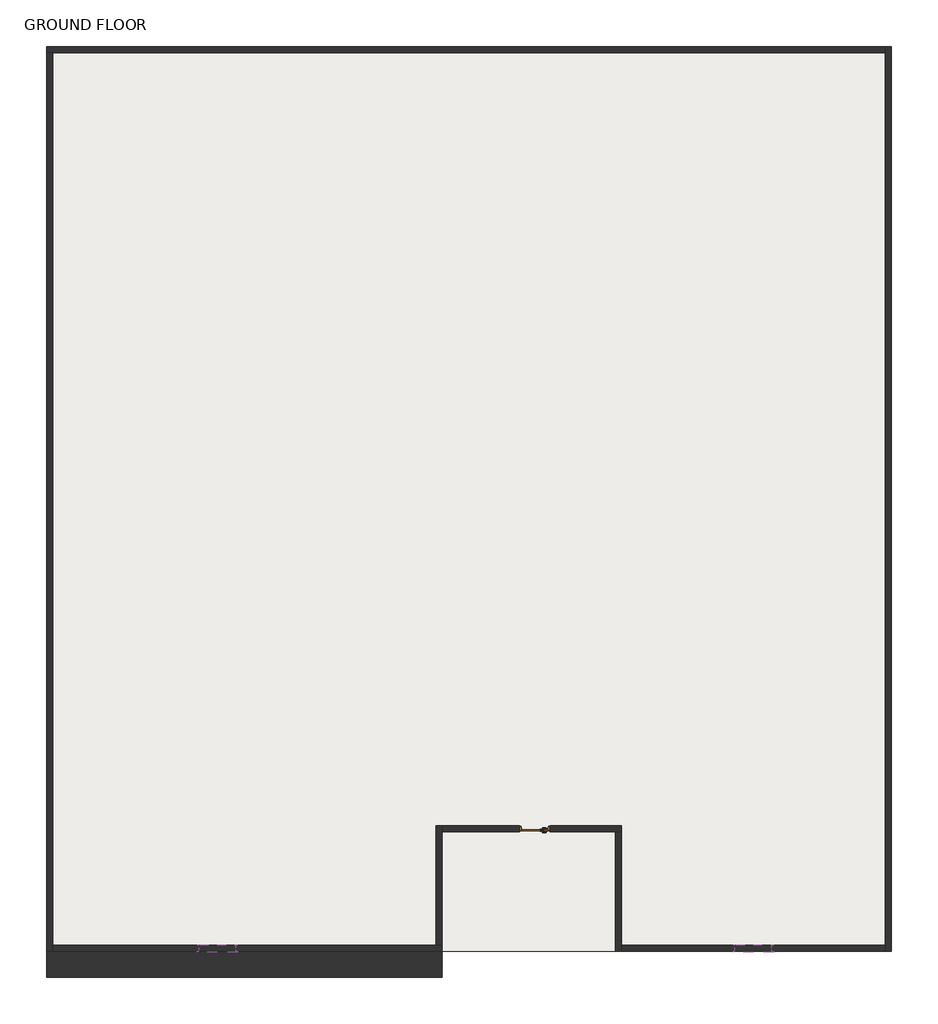
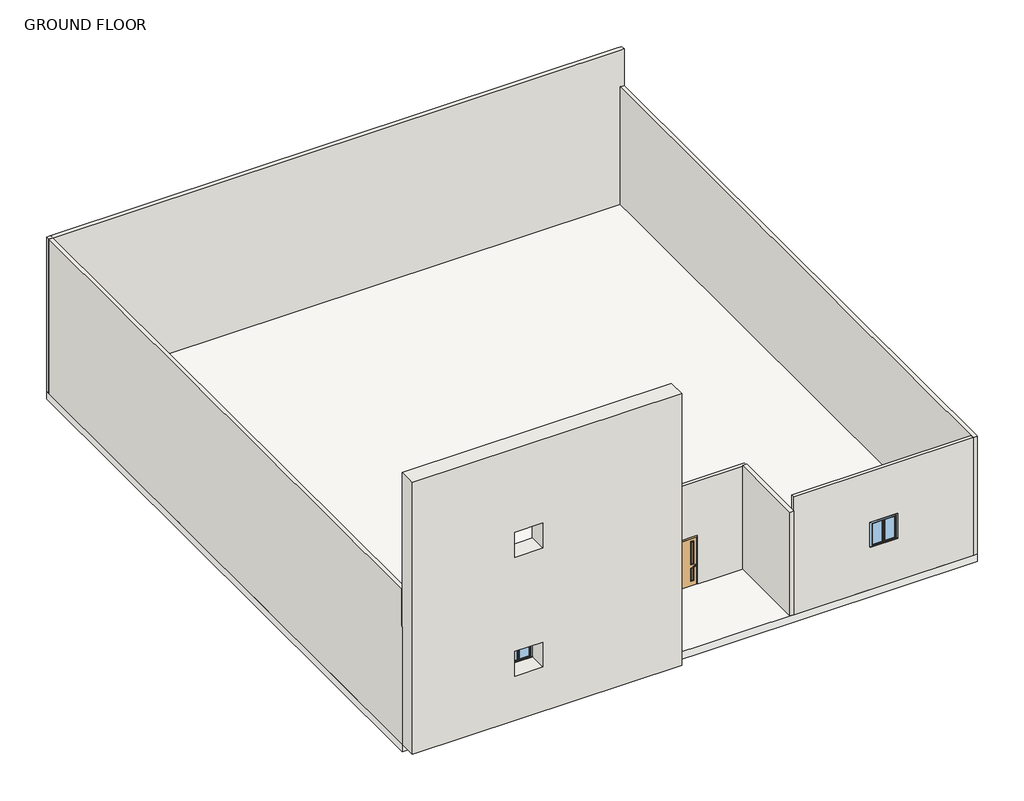
# One storey: 12 walls, 2 slabs, 2 windows, 1 door.
"""IFC4 building model written with IfcOpenShell, lengths in millimetres."""

from ifc_helpers import new_model, si_unit, frame, origin, place, context, project, spatial, polyline, outline, extrude, faceted_brep, transform, mapped, element, save
from components import door_81f4c142, walls_1_walls_1_ac0e2196, window_264d1730

model = new_model("IFC4")

# Units and contexts
model_context = context("Model", 3, world=origin())
ifc_project = project(units=[si_unit("LENGTHUNIT", "METRE", prefix="MILLI")], contexts=[model_context])

# Site, building, storey
site = spatial("IfcSite", under=ifc_project)
building = spatial("IfcBuilding", under=site)
storey = spatial("IfcBuildingStorey", under=building, Name="GROUND FLOOR", Elevation=0.0)

# Door
placement = place(None, origin())
door_shape = door_81f4c142(model_context)
element("IfcDoor", 1, ObjectType="Door-Passage-Single-Vision_Two_Lite : 36\" x 96\"", at=placement, inside=storey, context=model_context, shape_type="MappedRepresentation", body=[
    mapped(door_shape, transform((-1590.01982, -3826.5465627, 0.0), x_axis=(-1.0, 0.0, 0.0), y_axis=(0.0, -1.0, 0.0), z_axis=(0.0, 0.0, 1.0))),
])

# Slabs
element("IfcSlab", 2, ObjectType="Generic Floor - 400mm", at=placement, inside=storey, context=model_context, shape_type="SweptSolid", body=[
    extrude(outline(polyline([(10309.98018, 22267.1034373), (10309.98018, -7932.8965627), (-17890.01982, -7932.8965627), (-17890.01982, 22267.1034373), (10309.98018, 22267.1034373)])), frame((0.0, 0.0, -400.0), z_axis=(0.0, 0.0, 1.0), x_axis=(1.0, 0.0, 0.0)), (0.0, 0.0, 1.0), 400.0),
])
element("IfcSlab", 3, ObjectType="Generic Floor - 400mm", at=placement, inside=storey, context=model_context, shape_type="SweptSolid", body=[
    extrude(outline(polyline([(10309.98018, 22267.1034373), (10309.98018, -7932.8965627), (-17890.01982, -7932.8965627), (-17890.01982, 22267.1034373), (10309.98018, 22267.1034373)])), frame((0.0, 0.0, -400.0), z_axis=(0.0, 0.0, 1.0), x_axis=(1.0, 0.0, 0.0)), (0.0, 0.0, 1.0), 400.0),
])

# Walls
element("IfcWall", 4, ObjectType="Generic - 9\"", at=placement, inside=storey, context=model_context, shape_type="Brep", body=[
    faceted_brep([(-17890.01982, 22067.1034373, 8000.0), (-17890.01982, 22067.1034373, 6096.0), (-17890.01982, 22067.1034373, 0.0), (-17690.01982, 22067.1034373, 0.0), (10109.98018, 22067.1034373, 0.0), (10109.98018, 22067.1034373, 6096.0), (10309.98018, 22067.1034373, 6096.0), (10309.98018, 22067.1034373, 8000.0), (10109.98018, 22067.1034373, 8000.0), (-17690.01982, 22067.1034373, 8000.0), (-17890.01982, 22267.1034373, 0.0), (-17890.01982, 22267.1034373, 8000.0), (-17690.01982, 22267.1034373, 8000.0), (10109.98018, 22267.1034373, 8000.0), (10309.98018, 22267.1034373, 8000.0), (10309.98018, 22267.1034373, 6096.0), (10109.98018, 22267.1034373, 6096.0), (10109.98018, 22267.1034373, 0.0)], [[[0, 1, 2, 3, 4, 5, 6, 7, 8, 9]], [[10, 11, 12, 13, 14, 15, 16, 17]], [[4, 3, 2, 10, 17]], [[0, 9, 8, 7, 14, 13, 12, 11]], [[0, 11, 10, 2, 1]], [[15, 6, 5, 16]], [[5, 4, 17, 16]], [[7, 6, 15, 14]]]),
])
element("IfcWall", 5, ObjectType="Generic - 9\"", at=placement, inside=storey, context=model_context, shape_type="Brep", body=[
    faceted_brep([(-17690.01982, -7932.8965627, 0.0), (-17690.01982, -7732.8965627, 0.0), (-17690.01982, 22067.1034373, 0.0), (-17690.01982, 22067.1034373, 8000.0), (-17690.01982, -7832.8965627, 8000.0), (-17690.01982, -7832.8965627, 6096.0), (-17690.01982, -7932.8965627, 6096.0), (-17890.01982, -7932.8965627, 0.0), (-17890.01982, -7932.8965627, 6096.0), (-17890.01982, -7832.8965627, 6096.0), (-17890.01982, -7832.8965627, 8000.0), (-17890.01982, 22067.1034373, 8000.0), (-17890.01982, 22067.1034373, 0.0)], [[[0, 1, 2, 3, 4, 5, 6]], [[7, 8, 9, 10, 11, 12]], [[2, 1, 0, 7, 12]], [[4, 3, 11, 10]], [[5, 4, 10, 9]], [[5, 9, 8, 6]], [[0, 6, 8, 7]], [[2, 12, 11, 3]]]),
])
element("IfcWall", 6, ObjectType="Generic - 9\"", at=placement, inside=storey, context=model_context, shape_type="Brep", body=[
    faceted_brep([(10109.98018, 22267.1034373, 0.0), (10109.98018, 22067.1034373, 0.0), (10109.98018, -7732.8965627, 0.0), (10109.98018, -7932.8965627, 0.0), (10109.98018, -7932.8965627, 6096.0), (10109.98018, -7832.8965627, 6096.0), (10109.98018, -7732.8965627, 6096.0), (10109.98018, -3632.8965627, 6096.0), (10109.98018, 22067.1034373, 6096.0), (10109.98018, 22267.1034373, 6096.0), (10309.98018, 22267.1034373, 0.0), (10309.98018, 22267.1034373, 6096.0), (10309.98018, 22067.1034373, 6096.0), (10309.98018, -3632.8965627, 6096.0), (10309.98018, -7832.8965627, 6096.0), (10309.98018, -7932.8965627, 6096.0), (10309.98018, -7932.8965627, 0.0)], [[[0, 1, 2, 3, 4, 5, 6, 7, 8, 9]], [[10, 11, 12, 13, 14, 15, 16]], [[3, 2, 1, 0, 10, 16]], [[9, 8, 7, 6, 5, 4, 15, 14, 13, 12, 11]], [[0, 9, 11, 10]], [[4, 3, 16, 15]]]),
])
element("IfcWall", 7, ObjectType="Generic - 9\"", at=placement, inside=storey, context=model_context, shape_type="Brep", body=[
    faceted_brep([(-17690.01982, 22067.1034373, 8000.0), (-17690.01982, 22067.1034373, 0.0), (10109.98018, 22067.1034373, 0.0), (10109.98018, 22067.1034373, 6096.0), (10309.98018, 22067.1034373, 6096.0), (10309.98018, 22067.1034373, 8000.0), (10109.98018, 22067.1034373, 8000.0), (-17690.01982, 22267.1034373, 0.0), (-17690.01982, 22267.1034373, 8000.0), (10109.98018, 22267.1034373, 8000.0), (10309.98018, 22267.1034373, 8000.0), (10309.98018, 22267.1034373, 6096.0), (10109.98018, 22267.1034373, 6096.0), (10109.98018, 22267.1034373, 0.0)], [[[0, 1, 2, 3, 4, 5, 6]], [[7, 8, 9, 10, 11, 12, 13]], [[2, 1, 7, 13]], [[0, 6, 5, 10, 9, 8]], [[0, 8, 7, 1]], [[11, 4, 3, 12]], [[3, 2, 13, 12]], [[5, 4, 11, 10]]]),
])
element("IfcWall", 8, ObjectType="Generic - 9\"", at=placement, inside=storey, context=model_context, shape_type="Brep", body=[
    faceted_brep([(-17690.01982, -7932.8965627, 0.0), (-17690.01982, -7732.8965627, 0.0), (-17690.01982, 22067.1034373, 0.0), (-17690.01982, 22067.1034373, 8000.0), (-17690.01982, -7832.8965627, 8000.0), (-17690.01982, -7832.8965627, 6096.0), (-17690.01982, -7932.8965627, 6096.0), (-17890.01982, -7932.8965627, 0.0), (-17890.01982, -7932.8965627, 6096.0), (-17890.01982, -7832.8965627, 6096.0), (-17890.01982, -7832.8965627, 8000.0), (-17890.01982, 22067.1034373, 8000.0), (-17890.01982, 22067.1034373, 0.0)], [[[0, 1, 2, 3, 4, 5, 6]], [[7, 8, 9, 10, 11, 12]], [[2, 1, 0, 7, 12]], [[4, 3, 11, 10]], [[2, 12, 11, 3]], [[5, 4, 10, 9]], [[5, 9, 8, 6]], [[0, 6, 8, 7]]]),
])
element("IfcWall", 9, ObjectType="Generic - 9\"", at=placement, inside=storey, context=model_context, shape_type="Brep", body=[
    faceted_brep([(10109.98018, 22067.1034373, 0.0), (10109.98018, -7732.8965627, 0.0), (10109.98018, -7932.8965627, 0.0), (10109.98018, -7932.8965627, 6096.0), (10109.98018, -7832.8965627, 6096.0), (10109.98018, -7732.8965627, 6096.0), (10109.98018, -3632.8965627, 6096.0), (10109.98018, 22067.1034373, 6096.0), (10309.98018, 22067.1034373, 0.0), (10309.98018, 22067.1034373, 6096.0), (10309.98018, -3632.8965627, 6096.0), (10309.98018, -7832.8965627, 6096.0), (10309.98018, -7932.8965627, 6096.0), (10309.98018, -7932.8965627, 0.0)], [[[0, 1, 2, 3, 4, 5, 6, 7]], [[8, 9, 10, 11, 12, 13]], [[2, 1, 0, 8, 13]], [[7, 6, 5, 4, 3, 12, 11, 10, 9]], [[0, 7, 9, 8]], [[3, 2, 13, 12]]]),
])
element("IfcWall", 10, ObjectType="Generic - 9\"", at=placement, inside=storey, context=model_context, shape_type="Brep", body=[
    faceted_brep([(-17690.01982, -7932.8965627, 0.0), (-4690.01982, -7932.8965627, 0.0), (-4690.01982, -7932.8965627, 6096.0), (-4790.01982, -7932.8965627, 6096.0), (-17690.01982, -7932.8965627, 6096.0), (-12799.61982, -7932.8965627, 3545.6933591), (-11580.41982, -7932.8965627, 3545.6933591), (-11580.41982, -7932.8965627, 2326.4933591), (-12799.61982, -7932.8965627, 2326.4933591), (-17690.01982, -7732.8965627, 0.0), (-17690.01982, -7732.8965627, 6096.0), (-4790.01982, -7732.8965627, 6096.0), (-4690.01982, -7732.8965627, 6096.0), (-4690.01982, -7732.8965627, 5646.6011472), (-4690.01982, -7732.8965627, 0.0), (-4890.01982, -7732.8965627, 0.0), (-12799.61982, -7732.8965627, 3545.6933591), (-12799.61982, -7732.8965627, 2326.4933591), (-11580.41982, -7732.8965627, 2326.4933591), (-11580.41982, -7732.8965627, 3545.6933591), (-17690.01982, -7832.8965627, 6096.0)], [[[0, 1, 2, 3, 4], [5, 6, 7, 8]], [[9, 10, 11, 12, 13, 14, 15], [16, 17, 18, 19]], [[1, 0, 9, 15, 14]], [[4, 3, 2, 12, 11, 10, 20]], [[2, 1, 14, 13, 12]], [[0, 4, 20, 10, 9]], [[17, 16, 5, 8]], [[18, 17, 8, 7]], [[19, 18, 7, 6]], [[16, 19, 6, 5]]]),
])
element("IfcWall", 11, ObjectType="Generic - 9\"", at=placement, inside=storey, context=model_context, shape_type="Brep", body=[
    faceted_brep([(-4690.01982, -7732.8965627, 0.0), (-4690.01982, -3932.8965627, 0.0), (-4690.01982, -3732.8965627, 0.0), (-4690.01982, -3732.8965627, 5329.0930387), (-4690.01982, -3732.8965627, 5646.6011472), (-4690.01982, -7732.8965627, 5646.6011472), (-4890.01982, -7732.8965627, 0.0), (-4890.01982, -7732.8965627, 5646.6011472), (-4890.01982, -3732.8965627, 5646.6011472), (-4890.01982, -3732.8965627, 0.0)], [[[0, 1, 2, 3, 4, 5]], [[6, 7, 8, 9]], [[2, 1, 0, 6, 9]], [[5, 4, 8, 7]], [[0, 5, 7, 6]], [[4, 3, 2, 9, 8]]]),
])
element("IfcWall", 12, ObjectType="Generic - 9\"", at=placement, inside=storey, context=model_context, shape_type="Brep", body=[
    faceted_brep([(1309.98018, -3932.8965627, 5329.0930387), (-4690.01982, -3932.8965627, 5329.0930387), (-4690.01982, -3932.8965627, 0.0), (-2098.01982, -3932.8965627, 0.0), (-2098.01982, -3932.8965627, 2540.0), (-1082.01982, -3932.8965627, 2540.0), (-1082.01982, -3932.8965627, 0.0), (1109.98018, -3932.8965627, 0.0), (1309.98018, -3932.8965627, 0.0), (-4690.01982, -3732.8965627, 5329.0930387), (1309.98018, -3732.8965627, 5329.0930387), (1309.98018, -3732.8965627, 0.0), (-1082.01982, -3732.8965627, 0.0), (-1082.01982, -3732.8965627, 2540.0), (-2098.01982, -3732.8965627, 2540.0), (-2098.01982, -3732.8965627, 0.0), (-4690.01982, -3732.8965627, 0.0)], [[[0, 1, 2, 3, 4, 5, 6, 7, 8]], [[9, 10, 11, 12, 13, 14, 15, 16]], [[2, 16, 15, 3]], [[11, 8, 7, 6, 12]], [[1, 0, 10, 9]], [[2, 1, 9, 16]], [[0, 8, 11, 10]], [[14, 4, 3, 15]], [[4, 14, 13, 5]], [[5, 13, 12, 6]]]),
])
element("IfcWall", 13, ObjectType="Generic - 9\"", at=placement, inside=storey, context=model_context, shape_type="Brep", body=[
    faceted_brep([(1109.98018, -3932.8965627, 0.0), (1109.98018, -7932.8965627, 0.0), (1109.98018, -7932.8965627, 5381.5090557), (1109.98018, -3932.8965627, 5381.5090557), (1309.98018, -3932.8965627, 0.0), (1309.98018, -3932.8965627, 5329.0930387), (1309.98018, -3932.8965627, 5381.5090557), (1309.98018, -7932.8965627, 5381.5090557), (1309.98018, -7932.8965627, 0.0), (1309.98018, -7732.8965627, 0.0)], [[[0, 1, 2, 3]], [[4, 5, 6, 7, 8, 9]], [[1, 0, 4, 9, 8]], [[3, 2, 7, 6]], [[0, 3, 6, 5, 4]], [[2, 1, 8, 7]]]),
])
element("IfcWall", 14, ObjectType="Generic - 9\"", at=placement, inside=storey, context=model_context, shape_type="Brep", body=[
    faceted_brep([(1309.98018, -7932.8965627, 0.0), (10109.98018, -7932.8965627, 0.0), (10109.98018, -7932.8965627, 6096.0), (1309.98018, -7932.8965627, 6096.0), (1309.98018, -7932.8965627, 5381.5090557), (5100.38018, -7932.8965627, 3419.8751227), (6319.58018, -7932.8965627, 3419.8751227), (6319.58018, -7932.8965627, 2200.6751227), (5100.38018, -7932.8965627, 2200.6751227), (1309.98018, -7732.8965627, 0.0), (1309.98018, -7732.8965627, 6096.0), (10109.98018, -7732.8965627, 6096.0), (10109.98018, -7732.8965627, 0.0), (5100.38018, -7732.8965627, 3419.8751227), (5100.38018, -7732.8965627, 2200.6751227), (6319.58018, -7732.8965627, 2200.6751227), (6319.58018, -7732.8965627, 3419.8751227)], [[[0, 1, 2, 3, 4], [5, 6, 7, 8]], [[9, 10, 11, 12], [13, 14, 15, 16]], [[1, 0, 9, 12]], [[3, 2, 11, 10]], [[2, 1, 12, 11]], [[14, 13, 5, 8]], [[15, 14, 8, 7]], [[16, 15, 7, 6]], [[13, 16, 6, 5]], [[0, 4, 3, 10, 9]]]),
])
walls_1_walls_1_shape = walls_1_walls_1_ac0e2196(model_context)
element("IfcWall", 15, ObjectType="Walls 1 : Walls 1", at=placement, inside=storey, context=model_context, shape_type="MappedRepresentation", body=[
    mapped(walls_1_walls_1_shape, transform((0.0, 0.0, 0.0), x_axis=(1.0, 0.0, 0.0), y_axis=(0.0, 1.0, 0.0), z_axis=(0.0, 0.0, 1.0))),
])

# Windows
window_shape = window_264d1730(model_context)
element("IfcWindow", 16, ObjectType="Casement Dbl with Trim : 48\" x 48\"", at=placement, inside=storey, context=model_context, shape_type="MappedRepresentation", body=[
    mapped(window_shape, transform((-12190.01982, -7813.8465627, 1412.0933591), x_axis=(-1.0, 0.0, 0.0), y_axis=(0.0, -1.0, 0.0), z_axis=(0.0, 0.0, 1.0))),
])
element("IfcWindow", 17, ObjectType="Casement Dbl with Trim : 48\" x 48\"", at=placement, inside=storey, context=model_context, shape_type="MappedRepresentation", body=[
    mapped(window_shape, transform((5709.98018, -7813.8465627, 1286.2751227), x_axis=(-1.0, 0.0, 0.0), y_axis=(0.0, -1.0, 0.0), z_axis=(0.0, 0.0, 1.0))),
])

save(model, "model.ifc")

# Revit data of these elements
# Type "Door-Passage-Single-Vision_Two_Lite : 36\" x 96\""
#   Type Mark = "22"
#   Assembly Code = "B2030100"
#   Analytic Construction = "Wooden"
#   Thickness = 0' - 1 3/4"
#   Thermal Resistance (R) = 0.455703 (m²·K)/W
#   Swing Angle [instance default] = 90.00°
#   Strike Height = 3' - 4"
#   Rough Width [instance default] = 3' - 4"
#   Rough Height [instance default] = 8' - 4"
#   MF Opening Height [instance default] = 0' - 4"
#   MF Opening Width [instance default] = 0' - 4"
#   Heat Transfer Coefficient (U) = 2.19465 W/(m²·K)
#   Inset Calculate [instance default] = 0' - 4"
#   Masonry Inset [instance default] = 0' - 1"
#   Height = 8' - 0"
#   Width = 3' - 0"
#   Masonry Frame Depth = 0' - 5 3/4"
#   Masonry Frame [instance default] = yes
#   Function = 1
#   Dry Wall Frame [instance default] = no
#   Panel Material = Wood - Birch
#   Glazing = Glass
#   Glass Stop Material = Metal - Paint Finish - Grey
#   Frame Material = Metal - Paint Finish - Grey
#   Door Handle Material = Aluminum
#   Visual Light Transmittance = 0
#   Solar Heat Gain Coefficient = 0
#   Wall Closure = (empty or 0)
# Type "Generic Floor - 400mm"
#   Function = 0
#   Layers, outside or top first: 1' - 3.74803" no material (function 1)
# Type "Generic - 9\""
#   Layers, outside or top first: 0' - 7.87402" no material (function 1)
# Type "Casement Dbl with Trim : 48\" x 48\""
#   Type Mark = "19"
#   Construction Type Id = "GSP4R"
#   Assembly Code = "B2020100"
#   Analytic Construction = "1/8 in Pilkington single glazing"
#   Visual Light Transmittance = 0.9
#   Solar Heat Gain Coefficient = 0.78
#   Heat Transfer Coefficient (U) = 3.6886 W/(m²·K)
#   Height = 4' - 0"
#   Default Sill Height = 3' - 0"
#   Trim Projection - Ext. = 0' - 0 1/2"
#   Trim Projection - Int. = 0' - 0 3/4"
#   Trim Width - Exterior = 0' - 3 1/2"
#   Trim Width - Interior = 0' - 3 1/2"
#   Width = 4' - 0"
#   Window Inset = 0' - 0 3/4"
#   Define Thermal Properties by = 1
#   Glass Pane Material = Glass
#   Sash Material = Sash
#   Trim Exterior Material = Trim
#   Trim Interior Material = Trim
#   Wall Closure = (empty or 0)
# Element 1 (IfcDoor, "Door-Passage-Single-Vision_Two_Lite : 36\" x 96\"")
#   Swing Angle = 90.00°
#   Rough Width = 3' - 4"
#   Rough Height = 8' - 4"
#   Masonry Inset = 0' - 1"
#   MF Opening Width = 0' - 4"
#   MF Opening Height = 0' - 4"
#   Inset Calculate = 0' - 4"
#   Masonry Frame = yes
#   Dry Wall Frame = no
#   Phase Created = New Construction
#   Materials on its faces: "Metal - Paint Finish - Grey", "Aluminum", "Wood - Birch", "Glass"
# Elements 2, 3 (IfcSlab, "Generic Floor - 400mm")
#   Height Offset From Level = 0' - 0"
#   Phase Created = New Construction
#   Materials on its faces: "Default Roof"
# Elements 4, 5, 7, 8 (IfcWall, "Generic - 9\"")
#   Top Offset = 0' - 0"
#   Base Offset = 0' - 0"
#   Unconnected Height = 26' - 2.96063"
#   wall height = 26' - 2.96063"
#   Phase Created = New Construction
#   Base Constraint = GROUND FLOOR
#   Materials on its faces: "Default Wall"
# Elements 6, 9, 10, 14 (IfcWall, "Generic - 9\"")
#   Top Offset = 0' - 0"
#   Base Offset = 0' - 0"
#   Unconnected Height = 20' - 0"
#   wall height = 20' - 0"
#   Phase Created = New Construction
#   Base Constraint = GROUND FLOOR
#   Materials on its faces: "Default Wall"
# Element 11 (IfcWall, "Generic - 9\"")
#   Top Offset = 0' - 0"
#   Base Offset = 0' - 0"
#   Unconnected Height = 18' - 6.30713"
#   wall height = 18' - 6.30713"
#   Phase Created = New Construction
#   Base Constraint = GROUND FLOOR
#   Materials on its faces: "Default Wall"
# Element 12 (IfcWall, "Generic - 9\"")
#   Top Offset = 0' - 0"
#   Base Offset = 0' - 0"
#   Unconnected Height = 17' - 5.80681"
#   wall height = 17' - 5.80681"
#   Phase Created = New Construction
#   Base Constraint = GROUND FLOOR
#   Materials on its faces: "Default Wall"
# Element 13 (IfcWall, "Generic - 9\"")
#   Top Offset = 0' - 0"
#   Base Offset = 0' - 0"
#   Unconnected Height = 17' - 7.87044"
#   wall height = 17' - 7.87044"
#   Phase Created = New Construction
#   Base Constraint = GROUND FLOOR
#   Materials on its faces: "Default Wall"
# Element 15 (IfcWall, "Walls 1 : Walls 1")
#   Phase Created = New Construction
#   Materials on its faces: "Default Wall"
# Element 16 (IfcWindow, "Casement Dbl with Trim : 48\" x 48\"")
#   Mark = "6"
#   Phase Created = New Construction
#   Materials on its faces: "Sash", "Trim", "Glass"
# Element 17 (IfcWindow, "Casement Dbl with Trim : 48\" x 48\"")
#   Mark = "7"
#   Phase Created = New Construction
#   Materials on its faces: "Sash", "Trim", "Glass"
# Materials
#   "Wood - Birch": class "Wood", colour RGB 166 116 52, transparency 0, Cost = 0
#   "Glass": class "Glass", colour RGB 218 227 224, transparency 0.85, Description = "Soda Lime Glass", Cost = 0
#   "Metal - Paint Finish - Grey": class "Paint", colour RGB 104 104 104, transparency 0, Cost = 0
#   "Aluminum": class "Metal", colour RGB 244 244 244, transparency 0, Description = "Aluminum 6061", Cost = 0
#   "Sash": class "Wood", colour RGB 136 99 55, transparency 0
#   "Trim": class "Wood", colour RGB 224 178 126, transparency 0
#   "Default Roof": colour RGB 80 80 80, transparency 0
#   "Default Wall": colour RGB 80 80 80, transparency 0
